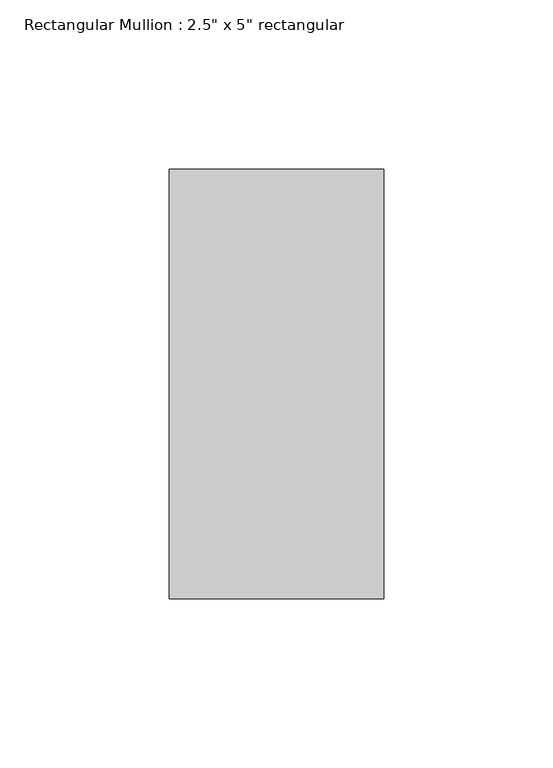
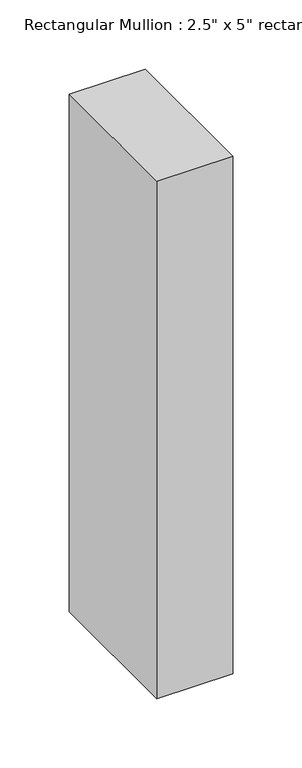
"""IFC4 building model written with IfcOpenShell, lengths in millimetres: member geometry."""

from ifc_helpers import new_model, si_unit, frame, origin, place, context, project, spatial, polyline, outline, extrude, source, transform, mapped, element, save


def member_15823cb3(model_context):
    return source(origin(), model_context, "Body", "SweptSolid", [
        extrude(outline(polyline([(0.0, 63.5), (0.0, -63.5), (-63.5, -63.5), (-63.5, 63.5), (0.0, 63.5)])), frame((0.0, 0.0, -457.2), z_axis=(0.0, 0.0, 1.0), x_axis=(1.0, 0.0, 0.0)), (0.0, 0.0, 1.0), 457.2),
    ])


if __name__ == "__main__":
    model = new_model("IFC4")
    model_context = context("Model", 3, world=origin())
    ifc_project = project(units=[si_unit("LENGTHUNIT", "METRE", prefix="MILLI")], contexts=[model_context])
    site = spatial("IfcSite", under=ifc_project)
    building = spatial("IfcBuilding", under=site)
    placement = place(None, origin())
    member_shape = member_15823cb3(model_context)
    element("IfcMember", 1, ObjectType="Rectangular Mullion : 2.5\" x 5\" rectangular", at=placement, inside=building, context=model_context, shape_type="MappedRepresentation", body=[
        mapped(member_shape, transform((0.0, 0.0, 0.0), x_axis=(1.0, 0.0, 0.0), y_axis=(0.0, 1.0, 0.0), z_axis=(0.0, 0.0, 1.0))),
    ])
    save(model, "model.ifc")

# Revit data of these elements
# Type "Rectangular Mullion : 2.5\" x 5\" rectangular"
#   built-in parameter 1007304 = 0.416667 (stored number, unit not read)
#   built-in parameter 1007301 = 0.104167 (stored number, unit not read)
#   built-in parameter 1007300 = 0.104167 (stored number, unit not read)
# Element 1 (IfcMember, "Rectangular Mullion : 2.5\" x 5\" rectangular")
#   Materials on its faces: "mullions"
# Materials
#   "mullions": class "Generic", colour RGB 120 120 120, transparency 0, Cost = 0
